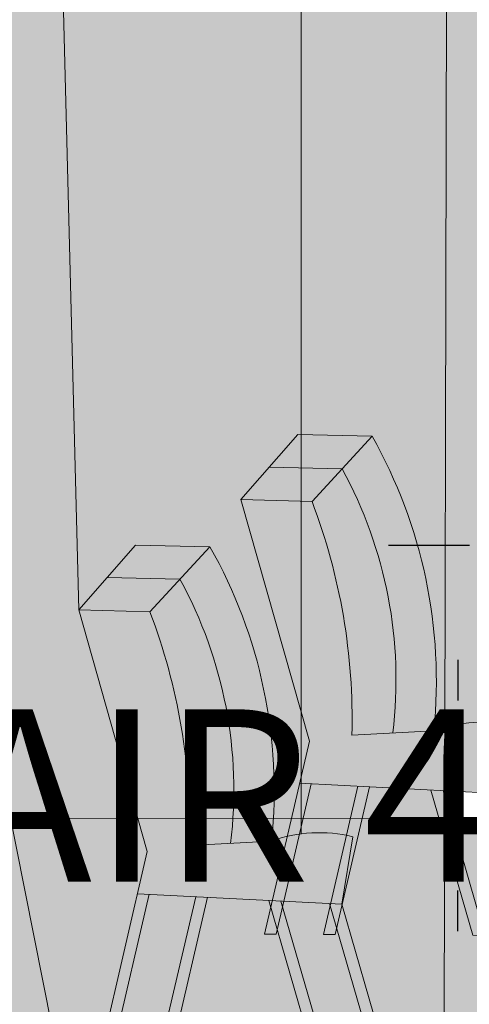
# Model space of a CAD drawing. Units: millimetres. Extents: x 11032 to 26788, y 3406 to 24505.
# Tile 6 of 78: x 15421 to 15812, y 7421 to 8278. Entities that reach past the tile are written whole.
import ezdxf

# ---------------------------------------------------------------- set-up
doc = ezdxf.new("R2010")
doc.units = ezdxf.units.MM
doc.header["$MEASUREMENT"] = 0
for name, color, linetype, lineweight in [('A-ANNO-DIMS', 2, 'Continuous', 18), ('A-FURN', 8, 'Continuous', 13), ('A-FURN-PATT', 8, 'Continuous', 13), ('A-GLAZ', 250, 'Continuous', 20), ('A-WALL-INTR', 8, 'Continuous', 18)]:
    doc.layers.add(name, color=color, linetype=linetype, lineweight=lineweight)
doc.layers.add('A-GLAZ-FRAM-PATT', color=250, linetype='Continuous', lineweight=13, true_color=0x262627)
doc.layers.add('A-WALL-INTR-PATT', color=251, linetype='Continuous', lineweight=13, true_color=0x6c6b6a)
doc.styles.get("Standard").update_dxf_attribs({"font": 'arial.ttf'})
doc.dimstyles.get("Standard").update_dxf_attribs({"dimtxt": 150, "dimasz": 100, "dimexe": 10, "dimexo": 5, "dimgap": 5, "dimtad": 0, "dimtih": 1, "dimtoh": 1, "dimdec": 0, "dimzin": 0, "dimdsep": 46, "dimtxsty": 'Standard', "dimcen": 0.09, "dimadec": 0, "dimazin": 0, "dimtfac": 1, "dimtdec": 0, "dimtofl": 0, "dimtmove": 0, "dimatfit": 3, "dimfxl": 1, "dimtolj": 1, "dimtzin": 0, "dimarcsym": 0})

# ---------------------------------------------------------------- blocks, each defined once
blk = doc.blocks.new('DINING-CHAIR-ELEV')
blk.add_line((228.68, 123.43), (51.04, 132.61))
for points in [[(0, 379.55), (49.45, 435.94), (114.12, 434.53)], [(61.18, 132.09), (30.79, 1.16), (20.53, 1.21), (59.55, 169.26), (0, 379.55), (61.9, 377.89)], [(111.9, 129.47), (82.06, 0.91), (71.8, 0.96), (101.76, 129.99)], [(165.28, 126.71), (201.76, 0.31), (212.19, 0.26), (175.85, 126.16)]]:
    blk.add_lwpolyline(points)
for points in [[(218.11, 123.98), (253.88, 0.05), (264.3, 0), (228.68, 123.43), (238.32, 182.18, 0.148451), (167.47, 178.33), (96.61, 174.48, 0.097012), (61.9, 377.89), (114.12, 434.53, -0.154833), (167.82, 178.46)], [(132.04, 176.4, 0.156877), (88.01, 406.21), (24.72, 407.74)]]:
    blk.add_lwpolyline(points, format="xyb")
blk = doc.blocks.new('*D16')
at = {"layer": 'A-ANNO-DIMS', "color": 0, "lineweight": -2, "transparency": 16777216}
for p, q in [((15741.74, 7821.05), (15812.13, 7821.05)), ((15802.13, 7721.05), (15802.13, 7685.69)), ((15802.13, 7485.11), (15802.13, 7520.47)), ((15741.74, 7385.11), (15812.13, 7385.11))]:
    blk.add_line(p, q, dxfattribs=at)
at = {"layer": 'A-ANNO-DIMS', "color": 0, "transparency": 16777216}
for points in [[(15785.47, 7721.05), (15818.8, 7721.05), (15802.13, 7821.05)], [(15785.47, 7485.11), (15818.8, 7485.11), (15802.13, 7385.11)]]:
    blk.add_solid(points, dxfattribs=at)
at = {"layer": 'Defpoints', "color": 0, "transparency": 16777216}
for p in [(15736.74, 7821.05), (15802.13, 7821.05), (15736.74, 7385.11)]:
    blk.add_point(p, dxfattribs=at)
at = {"layer": 'A-ANNO-DIMS', "color": 0, "transparency": 16777216, "insert": (15802.13, 7603.08), "char_height": 150, "attachment_point": 5}
blk.add_mtext('\\A1;CHAIR 436 TYP.', dxfattribs=at)
blk = doc.blocks.new('*D17')
at = {"layer": 'A-ANNO-DIMS', "color": 0, "lineweight": -2, "transparency": 16777216}
for p, q in [((15472.44, 7380.11), (15472.44, 7309.72)), ((15736.74, 7380.11), (15736.74, 7309.72)), ((15572.44, 7319.72), (15636.74, 7319.72)), ((15736.74, 7319.72), (15836.74, 7319.72))]:
    blk.add_line(p, q, dxfattribs=at)
at = {"layer": 'A-ANNO-DIMS', "color": 0, "transparency": 16777216}
for points in [[(15572.44, 7336.38), (15572.44, 7303.05), (15472.44, 7319.72)], [(15636.74, 7336.38), (15636.74, 7303.05), (15736.74, 7319.72)]]:
    blk.add_solid(points, dxfattribs=at)
at = {"layer": 'Defpoints', "color": 0, "transparency": 16777216}
for p in [(15472.44, 7385.11), (15736.74, 7385.11), (15736.74, 7319.72)]:
    blk.add_point(p, dxfattribs=at)
at = {"layer": 'A-ANNO-DIMS', "color": 0, "transparency": 16777216, "insert": (16266.37, 7319.72), "char_height": 150, "attachment_point": 5}
blk.add_mtext('\\A1;264 TYP.', dxfattribs=at)
blk = doc.blocks.new('*D36')
at = {"layer": 'A-ANNO-DIMS', "color": 0, "lineweight": -2, "transparency": 16777216}
for p, q in [((12301.26, 17115.89), (12301.26, 24416.86)), ((25397.4, 4466.4), (25397.4, 24416.86)), ((12401.26, 24406.86), (18569.2, 24406.86)), ((25297.4, 24406.86), (19129.47, 24406.86))]:
    blk.add_line(p, q, dxfattribs=at)
at = {"layer": 'A-ANNO-DIMS', "color": 0, "transparency": 16777216}
for points in [[(12401.26, 24423.52), (12401.26, 24390.19), (12301.26, 24406.86)], [(25297.4, 24423.52), (25297.4, 24390.19), (25397.4, 24406.86)]]:
    blk.add_solid(points, dxfattribs=at)
at = {"layer": 'Defpoints', "color": 0, "transparency": 16777216}
for p in [(25397.4, 24406.86), (12301.26, 17110.89), (25397.4, 4461.4)]:
    blk.add_point(p, dxfattribs=at)
at = {"layer": 'A-ANNO-DIMS', "color": 0, "transparency": 16777216, "insert": (18849.33, 24406.86), "char_height": 150, "attachment_point": 5}
blk.add_mtext('\\A1;13096', dxfattribs=at)
blk = doc.blocks.new('*D37')
at = {"layer": 'A-ANNO-DIMS', "color": 0, "lineweight": -2, "transparency": 16777216}
for p, q in [((18087.74, 23450.36), (11334.76, 23450.36)), ((11344.76, 23350.36), (11344.76, 14037.46)), ((11344.76, 4561.4), (11344.76, 13874.29)), ((12927.66, 4461.4), (11334.76, 4461.4))]:
    blk.add_line(p, q, dxfattribs=at)
at = {"layer": 'A-ANNO-DIMS', "color": 0, "transparency": 16777216}
for points in [[(11328.1, 23350.36), (11361.43, 23350.36), (11344.76, 23450.36)], [(11328.1, 4561.4), (11361.43, 4561.4), (11344.76, 4461.4)]]:
    blk.add_solid(points, dxfattribs=at)
at = {"layer": 'Defpoints', "color": 0, "transparency": 16777216}
for p in [(11344.76, 23450.36), (18092.74, 23450.36), (12932.66, 4461.4)]:
    blk.add_point(p, dxfattribs=at)
at = {"layer": 'A-ANNO-DIMS', "color": 0, "transparency": 16777216, "insert": (11344.76, 13955.88), "char_height": 150, "attachment_point": 5}
blk.add_mtext('\\A1;18989', dxfattribs=at)
blk = doc.blocks.new('*D49')
at = {"layer": 'A-ANNO-DIMS', "color": 0, "lineweight": -2, "transparency": 16777216}
for p, q in [((17953.45, 10206.41), (17953.45, 3494.9)), ((14996.4, 6406.4), (14996.4, 3494.9)), ((15096.4, 3504.9), (16244.67, 3504.9)), ((17853.45, 3504.9), (16705.18, 3504.9))]:
    blk.add_line(p, q, dxfattribs=at)
at = {"layer": 'A-ANNO-DIMS', "color": 0, "transparency": 16777216}
for points in [[(15096.4, 3521.57), (15096.4, 3488.23), (14996.4, 3504.9)], [(17853.45, 3521.57), (17853.45, 3488.23), (17953.45, 3504.9)]]:
    blk.add_solid(points, dxfattribs=at)
at = {"layer": 'Defpoints', "color": 0, "transparency": 16777216}
for p in [(17953.45, 10211.41), (14996.4, 6411.4), (17953.45, 3504.9)]:
    blk.add_point(p, dxfattribs=at)
at = {"layer": 'A-ANNO-DIMS', "color": 0, "transparency": 16777216, "insert": (16474.93, 3504.9), "char_height": 150, "attachment_point": 5}
blk.add_mtext('\\A1;2957', dxfattribs=at)
blk = doc.blocks.new('*D57')
at = {"layer": 'A-ANNO-DIMS', "color": 0, "lineweight": -2, "transparency": 16777216}
for p, q in [((14994.7, 7266.4), (14994.7, 24416.86)), ((20894.7, 7266.4), (20894.7, 24416.86)), ((15094.7, 24406.86), (17715.98, 24406.86)), ((20794.7, 24406.86), (18173.42, 24406.86))]:
    blk.add_line(p, q, dxfattribs=at)
at = {"layer": 'A-ANNO-DIMS', "color": 0, "transparency": 16777216}
for points in [[(15094.7, 24423.52), (15094.7, 24390.19), (14994.7, 24406.86)], [(20794.7, 24423.52), (20794.7, 24390.19), (20894.7, 24406.86)]]:
    blk.add_solid(points, dxfattribs=at)
at = {"layer": 'Defpoints', "color": 0, "transparency": 16777216}
for p in [(20894.7, 24406.86), (14994.7, 7261.4), (20894.7, 7261.4)]:
    blk.add_point(p, dxfattribs=at)
at = {"layer": 'A-ANNO-DIMS', "color": 0, "transparency": 16777216, "insert": (17944.7, 24406.86), "char_height": 150, "attachment_point": 5}
blk.add_mtext('\\A1;5900', dxfattribs=at)
blk = doc.blocks.new('*D60')
at = {"layer": 'A-ANNO-DIMS', "color": 0, "lineweight": -2, "transparency": 16777216}
for p, q in [((14994.7, 7266.4), (14994.7, 24416.86)), ((16344.7, 7266.4), (16344.7, 24416.86)), ((15094.7, 24406.86), (15448.04, 24406.86)), ((16244.7, 24406.86), (15891.36, 24406.86))]:
    blk.add_line(p, q, dxfattribs=at)
at = {"layer": 'A-ANNO-DIMS', "color": 0, "transparency": 16777216}
for points in [[(15094.7, 24423.52), (15094.7, 24390.19), (14994.7, 24406.86)], [(16244.7, 24423.52), (16244.7, 24390.19), (16344.7, 24406.86)]]:
    blk.add_solid(points, dxfattribs=at)
at = {"layer": 'Defpoints', "color": 0, "transparency": 16777216}
for p in [(16344.7, 24406.86), (14994.7, 7261.4), (16344.7, 7261.4)]:
    blk.add_point(p, dxfattribs=at)
at = {"layer": 'A-ANNO-DIMS', "color": 0, "transparency": 16777216, "insert": (15669.7, 24406.86), "char_height": 150, "attachment_point": 5}
blk.add_mtext('\\A1;1350', dxfattribs=at)
blk = doc.blocks.new('*D69')
at = {"layer": 'A-ANNO-DIMS', "color": 0, "lineweight": -2, "transparency": 16777216}
for p, q in [((13956.97, 9937.95), (14056.97, 9937.95)), ((14056.97, 9937.95), (15432.5, 8990.95)), ((17944.61, 7261.4), (17944.79, 7261.4)), ((17944.7, 7261.31), (17944.7, 7261.49))]:
    blk.add_line(p, q, dxfattribs=at)
at = {"layer": 'A-ANNO-DIMS', "color": 0, "transparency": 16777216}
blk.add_solid([(15441.95, 9004.68), (15423.05, 8977.22), (15514.87, 8934.24)], dxfattribs=at)
at = {"layer": 'Defpoints', "color": 0, "transparency": 16777216}
for p in [(15514.87, 8934.24), (17944.7, 7261.4)]:
    blk.add_point(p, dxfattribs=at)
at = {"layer": 'A-ANNO-DIMS', "color": 0, "transparency": 16777216, "insert": (13494.04, 9937.95), "char_height": 150, "attachment_point": 5}
blk.add_mtext('\\A1;2X R2950', dxfattribs=at)

msp = doc.modelspace()

# ---------------------------------------------------------------- hatches: boundary and pattern name
at = {"layer": 'A-FURN-PATT'}
h = msp.add_hatch(color=256, dxfattribs=at)
h.set_gradient(color1=(153, 27, 30), color2=(153, 38, 0), name='SPHERICAL')
h.paths.add_polyline_path([(15534.344, 7763), (15472.44, 7764.657), (15531.986, 7554.365), (15523.479, 7517.719), (15640.736, 7511.661), (15653.713, 7567.556, 0.0295203), (15639.906, 7563.436), (15569.055, 7559.583, 0.0970121)], flags=16)
h.paths.add_polyline_path([(15560.453, 7791.32), (15534.344, 7763, -0.0970121), (15569.055, 7559.583), (15604.48, 7561.509, 0.1568775)], flags=16)
h.paths.add_polyline_path([(15586.562, 7819.64), (15560.453, 7791.32, -0.1568775), (15604.48, 7561.509), (15640.246, 7563.454, 0.154898)], flags=17)
h.paths.add_polyline_path([(15560.453, 7791.32), (15497.165, 7792.851), (15472.44, 7764.657), (15534.344, 7763)], flags=16)
h.paths.add_polyline_path([(15586.562, 7819.64), (15521.889, 7821.046), (15497.165, 7792.851), (15560.453, 7791.32)], flags=17)
h.paths.add_polyline_path([(15790.874, 7662.689, 0.021469), (15780.879, 7659.53), (15710.028, 7655.677, 0.0970121), (15675.317, 7859.094), (15665.772, 7859.35), (15665.799, 7675.745), (15672.959, 7650.459), (15665.807, 7619.654), (15665.808, 7613.744), (15790.755, 7607.288)], flags=17)
h.paths.add_polyline_path([(15665.772, 7859.35), (15613.413, 7860.751), (15665.799, 7675.745)], flags=16)
h.paths.add_polyline_path([(15701.426, 7887.414), (15665.767, 7888.277), (15665.772, 7859.35), (15675.317, 7859.094)], flags=16)
h.paths.add_polyline_path([(15727.534, 7915.735), (15665.763, 7917.077), (15665.767, 7888.277), (15701.426, 7887.414)], flags=17)
h.paths.add_polyline_path([(15665.763, 7917.077), (15662.862, 7917.14), (15638.137, 7888.946), (15665.767, 7888.277)], flags=17)
h.paths.add_polyline_path([(15665.767, 7888.277), (15638.137, 7888.946), (15613.413, 7860.751), (15665.772, 7859.35)], flags=16)
h.paths.add_polyline_path([(15701.426, 7887.414), (15675.317, 7859.094, -0.0970121), (15710.028, 7655.677), (15745.453, 7657.604, 0.1568775)], flags=16)
h.paths.add_polyline_path([(15844.495, 7664.925), (15844.384, 7864.461), (15821.312, 7945.94), (15870.762, 8002.329), (15935.434, 8000.923, -0.1195917), (15991.005, 7804.617), (16002.667, 7804.617), (16022.264, 7889.032), (15962.718, 8099.323), (16024.622, 8097.666), (16076.839, 8154.307, -0.1548334), (16130.535, 7898.229, -0.1476694), (16201.035, 7901.954), (16191.395, 7843.208), (16202.533, 7804.617), (16299.12, 7804.617), (16297.929, 7808.825), (16347.378, 7865.214), (16412.05, 7863.808, -0.0295496), (16434.494, 7817.915), (16458.237, 7920.19), (16398.691, 8130.481), (16460.595, 8128.825), (16512.813, 8185.465, -0.1548334), (16566.508, 7929.387, -0.1476694), (16637.008, 7933.112), (16627.369, 7874.366), (16647.499, 7804.617), (16830.506, 7804.617), (16830.506, 7793.515), (16650.704, 7793.515), (16662.994, 7750.932), (16652.571, 7750.983), (16640.296, 7793.515), (16490.425, 7793.515), (16480.749, 7751.837), (16470.495, 7751.888), (16480.159, 7793.515), (16443.833, 7793.515, -0.1094051), (16465.746, 7607.731, -0.1476694), (16536.246, 7611.456), (16526.606, 7552.71), (16562.232, 7429.275), (16551.809, 7429.327), (16516.041, 7553.255), (16473.778, 7555.439), (16510.116, 7429.534), (16499.693, 7429.586), (16463.212, 7555.985), (16409.833, 7558.743), (16379.987, 7430.181), (16369.733, 7430.232), (16394.704, 7537.793), (16394.704, 7559.524), (16359.112, 7561.363), (16328.717, 7430.435), (16318.463, 7430.486), (16344.704, 7543.521), (16344.704, 7643.635), (16302.264, 7793.515), (16205.738, 7793.515), (16227.021, 7719.773), (16216.598, 7719.825), (16195.329, 7793.515), (16153.697, 7793.515), (16174.905, 7720.032), (16164.482, 7720.084), (16143.289, 7793.515), (16061.685, 7793.515), (16051.641, 7750.248, -0.0167144), (16059.629, 7748.571), (16049.99, 7689.825), (16085.615, 7566.39), (16075.192, 7566.442), (16039.424, 7690.371), (15997.161, 7692.554), (16033.5, 7566.649), (16023.077, 7566.701), (15986.595, 7693.1), (15933.216, 7695.858), (15903.371, 7567.296), (15893.116, 7567.347), (15923.072, 7696.382), (15882.495, 7698.478), (15852.409, 7568.882), (15877.716, 7481.201), (15867.293, 7481.253), (15842.372, 7567.599), (15841.846, 7567.602), (15842.08, 7568.609), (15831.524, 7605.182), (15790.755, 7607.288), (15790.744, 7602.228), (15825.6, 7481.46), (15815.177, 7481.512), (15778.696, 7607.911), (15725.317, 7610.669), (15701.389, 7507.6), (15736.743, 7385.107), (15726.32, 7385.159), (15696.749, 7487.614), (15695.471, 7482.107), (15685.217, 7482.158), (15691.06, 7507.327), (15690.552, 7509.088), (15650.881, 7511.137), (15649.743, 7506.234), (15684.627, 7385.366), (15674.204, 7385.418), (15645.103, 7486.248), (15644.2, 7482.362), (15633.946, 7482.413), (15639.413, 7505.961), (15637.723, 7511.817), (15584.344, 7514.575), (15554.498, 7386.013), (15544.244, 7386.064), (15574.2, 7515.099), (15533.623, 7517.195), (15503.228, 7386.268), (15492.974, 7386.319), (15531.986, 7554.365), (15472.44, 7764.657), (15497.165, 7792.851), (15521.889, 7821.046), (15586.562, 7819.64, -0.1548334), (15640.257, 7563.563, -0.0287549), (15653.713, 7567.556), (15665.807, 7619.654), (15665.799, 7675.745), (15613.413, 7860.751), (15638.137, 7888.946), (15662.862, 7917.14), (15665.763, 7917.077), (15727.534, 7915.735, -0.1548334), (15781.23, 7659.657, -0.1322263)])
h = msp.add_hatch(color=256, dxfattribs=at)
h.set_gradient(color1=(153, 27, 30), color2=(153, 38, 0), name='SPHERICAL')
h.paths.add_polyline_path([(15710.028, 7655.677), (15745.453, 7657.604, 0.1568775), (15701.426, 7887.414), (15675.317, 7859.094, -0.0970121)], flags=16)
h.paths.add_polyline_path([(15790.755, 7607.288), (15790.874, 7662.689, 0.021469), (15780.879, 7659.53), (15710.028, 7655.677, 0.0970121), (15675.317, 7859.094), (15665.772, 7859.35), (15665.799, 7675.745), (15672.959, 7650.459), (15665.807, 7619.654), (15665.808, 7613.744)], flags=17)
h.paths.add_polyline_path([(15653.713, 7567.556), (15665.807, 7619.654), (15665.799, 7675.745), (15613.413, 7860.751), (15662.862, 7917.14), (15727.534, 7915.735, -0.1548334), (15781.23, 7659.657, -0.1322263), (15844.495, 7664.925), (15844.384, 7864.461), (15821.312, 7945.94), (15883.216, 7944.283), (15935.434, 8000.923, -0.1195917), (15991.005, 7804.617), (16002.667, 7804.617), (16022.264, 7889.032), (15962.718, 8099.323), (16024.622, 8097.666), (16076.839, 8154.307, -0.1548334), (16130.535, 7898.229, -0.1476694), (16201.035, 7901.954), (16191.395, 7843.208), (16202.533, 7804.617), (16830.506, 7804.617), (16830.506, 7793.515), (16205.738, 7793.515), (16227.021, 7719.773), (16216.598, 7719.825), (16195.329, 7793.515), (16153.697, 7793.515), (16174.905, 7720.032), (16164.482, 7720.084), (16143.289, 7793.515), (16061.685, 7793.515), (16051.641, 7750.248, -0.0167144), (16059.629, 7748.571), (16049.99, 7689.825), (16085.615, 7566.39), (16075.192, 7566.442), (16039.424, 7690.371), (15997.161, 7692.554), (16033.5, 7566.649), (16023.077, 7566.701), (15986.595, 7693.1), (15933.216, 7695.858), (15903.371, 7567.296), (15893.116, 7567.347), (15923.072, 7696.382), (15882.495, 7698.478), (15852.409, 7568.882), (15877.716, 7481.201), (15867.293, 7481.253), (15842.372, 7567.599), (15841.846, 7567.602), (15842.08, 7568.609), (15831.524, 7605.182), (15790.755, 7607.288), (15790.744, 7602.228), (15825.6, 7481.46), (15815.177, 7481.512), (15778.696, 7607.911), (15725.317, 7610.669), (15701.389, 7507.6), (15736.743, 7385.107), (15726.32, 7385.159), (15696.749, 7487.614), (15695.471, 7482.107), (15685.217, 7482.158), (15705.262, 7568.502, 0.0841685), (15664.448, 7569.579), (15644.2, 7482.362), (15633.946, 7482.413), (15653.713, 7567.556, 0.0295203), (15639.906, 7563.436), (15569.055, 7559.583, 0.0970121), (15534.344, 7763), (15472.44, 7764.657), (15521.889, 7821.046), (15586.562, 7819.64, -0.1548334), (15640.257, 7563.563, -0.0287549)])
h = msp.add_hatch(color=256, dxfattribs=at)
h.set_gradient(color1=(153, 27, 30), color2=(153, 38, 0), name='SPHERICAL')
h.paths.add_polyline_path([(15675.317, 7859.094), (15665.772, 7859.35), (15665.799, 7675.745), (15672.959, 7650.459), (15665.807, 7619.654), (15665.808, 7613.744), (15790.755, 7607.288), (15790.874, 7662.689, 0.021469), (15780.879, 7659.53), (15710.028, 7655.677, 0.0970121)])
h.paths.add_polyline_path([(15710.028, 7655.677), (15745.453, 7657.604, 0.1568775), (15701.426, 7887.414), (15675.317, 7859.094, -0.0970121)])
h = msp.add_hatch(color=256, dxfattribs=at)
h.set_gradient(color1=(153, 27, 30), color2=(153, 38, 0), name='SPHERICAL')
h.paths.add_polyline_path([(15534.344, 7763), (15472.44, 7764.657), (15531.986, 7554.365), (15523.479, 7517.719), (15640.736, 7511.661), (15653.713, 7567.556, 0.0295203), (15639.906, 7563.436), (15569.055, 7559.583, 0.0970121)])
h.paths.add_polyline_path([(15560.453, 7791.32), (15534.344, 7763, -0.0970121), (15569.055, 7559.583), (15604.48, 7561.509, 0.1568775)])
at = {"layer": 'A-GLAZ-FRAM-PATT'}
h = msp.add_hatch(color=256, dxfattribs=at)
h.paths.add_polyline_path([(17944.704, 7311.399), (16344.704, 7311.399), (16344.704, 7261.399), (17944.704, 7261.399)], flags=17)
h.paths.add_polyline_path([(16344.704, 7311.399), (15045.135, 7311.399, -0.9829047), (20844.273, 7311.399), (19544.704, 7311.399), (19544.704, 7261.399), (20894.704, 7261.399, 0.5148441), (16985.951, 10051.255, 0.3202679), (14994.704, 7261.399), (16344.704, 7261.399)])
h.paths.add_polyline_path([(18744.704, 7311.399), (17944.704, 7311.399), (17944.704, 7261.399), (18744.704, 7261.399)], flags=17)
h.paths.add_polyline_path([(19544.704, 7311.399), (18744.704, 7311.399), (18744.704, 7261.399), (19544.704, 7261.399)], flags=17)
h.paths.add_polyline_path([(18694.704, 7361.399), (17994.704, 7361.399), (17994.704, 7311.399), (18694.704, 7311.399)], flags=17)
h.paths.add_polyline_path([(18744.704, 7361.399), (18694.704, 7361.399), (18694.704, 7311.399), (18744.704, 7311.399)], flags=17)
h.paths.add_polyline_path([(17194.704, 7361.399), (17144.704, 7361.399), (17144.704, 7311.399), (17194.704, 7311.399)], flags=17)
h.paths.add_polyline_path([(17431.432, 7361.399), (17194.704, 7361.399), (17194.704, 7311.399), (17431.699, 7311.399)], flags=17)
h.paths.add_polyline_path([(17894.704, 7361.399), (17431.432, 7361.399), (17431.699, 7311.399), (17894.704, 7311.399)], flags=17)
h.paths.add_polyline_path([(17944.704, 7361.399), (17894.704, 7361.399), (17894.704, 7311.399), (17944.704, 7311.399)], flags=17)
h.paths.add_polyline_path([(17994.704, 7361.399), (17944.704, 7361.399), (17944.704, 7311.399), (17994.704, 7311.399)], flags=17)
at = {"layer": 'A-WALL-INTR-PATT'}
for points in [[(15843.607, 9260.247, 0.0062633), (15794.195, 9206.987), (15790.874, 7662.689, -0.1112179), (15844.495, 7664.925), (15844.384, 7864.461), (15821.312, 7945.94), (15844.324, 7972.181)], [(15794.195, 9206.987, 0.0171928), (15665.595, 9054.627), (15665.763, 7917.077), (15727.534, 7915.735, -0.1548334), (15781.23, 7659.657, -0.0207039), (15790.874, 7662.689)], [(15665.595, 9054.627, 0.0332657), (15447.906, 8736.527), (15472.44, 7764.657), (15521.889, 7821.046), (15586.562, 7819.64, -0.1548334), (15640.257, 7563.563, -0.0287549), (15653.713, 7567.556), (15665.807, 7619.654), (15665.799, 7675.745), (15613.413, 7860.751), (15662.862, 7917.14), (15665.763, 7917.077)], [(15447.906, 8736.527, 0.0271717), (15302.659, 8457.059), (15381.661, 7740.545), (15467.334, 7311.399), (15790.119, 7311.399), (15790.667, 7566.433), (15778.696, 7607.911), (15725.317, 7610.669), (15701.389, 7507.6), (15736.743, 7385.107), (15726.32, 7385.159), (15696.749, 7487.614), (15695.471, 7482.107), (15685.217, 7482.158), (15691.06, 7507.327), (15690.552, 7509.088), (15650.881, 7511.137), (15649.743, 7506.234), (15684.627, 7385.366), (15674.204, 7385.418), (15645.103, 7486.248), (15644.2, 7482.362), (15633.946, 7482.413), (15639.413, 7505.961), (15637.723, 7511.817), (15584.344, 7514.575), (15554.498, 7386.013), (15544.244, 7386.064), (15574.2, 7515.099), (15533.623, 7517.195), (15503.228, 7386.268), (15492.974, 7386.319), (15531.986, 7554.365), (15472.44, 7764.657)]]:
    msp.add_hatch(color=256, dxfattribs=at).paths.add_polyline_path(points)
h = msp.add_hatch(color=256, dxfattribs=at)
h.paths.add_polyline_path([(15302.659, 8457.059, 0.0281002), (15185.248, 8153.253), (15233.282, 7717.599), (15314.374, 7311.399), (15467.334, 7311.399), (15381.661, 7740.545)])
h.paths.add_polyline_path([(16344.704, 7543.521), (16344.704, 7643.635), (16302.264, 7793.515), (16205.738, 7793.515), (16227.021, 7719.773), (16216.598, 7719.825), (16195.329, 7793.515), (16153.697, 7793.515), (16174.905, 7720.032), (16164.482, 7720.084), (16143.289, 7793.515), (16061.685, 7793.515), (16051.641, 7750.248, -0.0167144), (16059.629, 7748.571), (16049.99, 7689.825), (16085.615, 7566.39), (16075.192, 7566.442), (16039.424, 7690.371), (15997.161, 7692.554), (16033.5, 7566.649), (16023.077, 7566.701), (15986.595, 7693.1), (15933.216, 7695.858), (15903.371, 7567.296), (15893.116, 7567.347), (15923.072, 7696.382), (15882.495, 7698.478), (15852.409, 7568.882), (15877.716, 7481.201), (15867.293, 7481.253), (15844.553, 7560.041), (15844.691, 7311.399), (16344.704, 7311.399), (16344.704, 7499.3), (16328.717, 7430.435), (16318.463, 7430.486)])
h.paths.add_polyline_path([(16742.983, 7793.515), (16650.704, 7793.515), (16662.994, 7750.932), (16652.571, 7750.983), (16640.296, 7793.515), (16598.663, 7793.515), (16610.879, 7751.191), (16600.455, 7751.242), (16588.255, 7793.515), (16490.425, 7793.515), (16480.749, 7751.837), (16470.495, 7751.888), (16480.159, 7793.515), (16443.833, 7793.515, -0.1094051), (16465.746, 7607.731, -0.1476694), (16536.246, 7611.456), (16526.606, 7552.71), (16562.232, 7429.275), (16551.809, 7429.327), (16516.041, 7553.255), (16473.778, 7555.439), (16510.116, 7429.534), (16499.693, 7429.586), (16463.212, 7555.985), (16409.833, 7558.743), (16394.704, 7493.572), (16394.704, 7361.399), (16744.704, 7361.399)])
h.paths.add_polyline_path([(17094.704, 8239.696), (16741.207, 8239.696), (16742.939, 7804.617), (16768.057, 7804.617), (16785.352, 7864.542), (16775.713, 7923.288, -0.1476694), (16846.212, 7919.563, -0.1548334), (16899.908, 8175.64), (16964.58, 8177.046), (17014.03, 8120.657), (16954.484, 7910.365), (16972.017, 7834.84), (16977.75, 7834.965), (17027.199, 7778.576), (16967.653, 7568.284), (17006.665, 7400.238), (16996.411, 7400.187), (16966.016, 7531.114), (16925.439, 7529.018), (16955.395, 7399.983), (16945.141, 7399.932), (16915.295, 7528.494), (16861.916, 7525.736), (16825.435, 7399.337), (16815.012, 7399.285), (16851.35, 7525.19), (16809.087, 7523.007), (16773.319, 7399.078), (16762.896, 7399.026), (16798.521, 7522.461), (16788.882, 7581.207, -0.1476694), (16859.382, 7577.482, -0.1528132), (16911.41, 7830.579), (16902.125, 7870.575), (16848.746, 7867.817), (16830.506, 7804.617), (16830.506, 7793.515), (16827.302, 7793.515), (16812.265, 7741.418), (16801.842, 7741.366), (16816.893, 7793.515), (16775.261, 7793.515), (16760.15, 7741.159), (16749.727, 7741.107), (16764.853, 7793.515), (16742.983, 7793.515), (16744.704, 7361.399), (17094.704, 7361.399)])
h.paths.add_polyline_path([(18950.929, 7931.023), (19015.601, 7932.429), (19065.05, 7876.04), (19005.504, 7665.748), (19014.012, 7629.102, -0.129191), (19069.892, 7841.762), (19134.564, 7843.167), (19168.958, 7803.946), (19202.145, 7841.791), (19246.92, 7840.817), (19212.932, 7960.847), (19262.382, 8017.236), (19327.054, 8015.831, -0.134919), (19382.824, 7793.43), (19562.845, 7793.43, -0.1257757), (19618.686, 8000.275), (19683.358, 8001.68), (19732.808, 7945.291), (19689.807, 7793.43), (19753.644, 7793.43, -0.0966843), (19805.964, 7950.707), (19870.637, 7952.112), (19920.086, 7895.723), (19891.121, 7793.43), (20039.255, 7793.43, -0.0897865), (20089.9, 7938.993), (20154.572, 7940.399), (20204.021, 7884.01), (20144.475, 7673.718), (20152.983, 7637.072, -0.1476694), (20223.483, 7633.347, -0.1548334), (20277.178, 7889.425), (20341.85, 7890.831), (20391.3, 7834.441), (20331.754, 7624.15), (20370.766, 7456.103), (20360.512, 7456.052), (20330.117, 7586.98), (20289.54, 7584.884), (20319.496, 7455.848), (20309.241, 7455.797), (20279.396, 7584.359), (20226.017, 7581.602), (20189.536, 7455.202), (20179.112, 7455.151), (20215.451, 7581.056), (20173.188, 7578.872), (20169.478, 7566.018), (20183.488, 7505.671), (20173.234, 7505.62), (20163.789, 7546.305), (20137.42, 7454.943), (20126.997, 7454.892), (20159.149, 7566.291), (20142.839, 7636.548), (20102.261, 7634.452), (20132.217, 7505.417), (20121.963, 7505.366), (20092.117, 7633.928), (20038.738, 7631.17), (20002.257, 7504.771), (19991.834, 7504.719), (20028.172, 7630.624), (19985.91, 7628.44), (19950.141, 7504.512), (19939.718, 7504.46), (19975.344, 7627.895), (19965.704, 7686.641, -0.1476694), (20036.204, 7682.916, -0.0576487), (20037.659, 7782.328), (19887.977, 7782.328), (19860.54, 7685.431), (19899.552, 7517.385), (19889.298, 7517.334), (19858.903, 7648.261), (19818.326, 7646.165), (19848.282, 7517.13), (19838.028, 7517.079), (19808.182, 7645.641), (19754.803, 7642.883), (19718.322, 7516.484), (19707.899, 7516.432), (19744.237, 7642.337), (19701.974, 7640.154), (19698.264, 7627.3), (19712.274, 7566.953), (19702.02, 7566.902), (19692.575, 7607.587), (19666.206, 7516.225), (19655.783, 7516.173), (19687.935, 7627.573), (19671.625, 7697.83), (19631.048, 7695.733), (19661.003, 7566.698), (19650.749, 7566.647), (19620.903, 7695.209), (19567.524, 7692.451), (19531.043, 7566.052), (19520.62, 7566), (19556.959, 7691.905), (19514.696, 7689.722), (19478.928, 7565.793), (19468.505, 7565.741), (19473, 7581.318), (19466.812, 7581.349), (19431.044, 7705.278), (19388.781, 7707.461), (19425.12, 7581.556), (19414.696, 7581.608), (19378.215, 7708.007), (19324.836, 7710.765), (19318.877, 7685.094, -0.0584523), (19320.513, 7584.307, -0.1476694), (19391.013, 7588.032), (19381.373, 7529.286), (19416.999, 7405.852), (19406.576, 7405.903), (19370.808, 7529.832), (19328.545, 7532.016), (19364.883, 7406.111), (19354.46, 7406.162), (19317.979, 7532.562), (19264.6, 7535.319), (19234.754, 7406.757), (19224.5, 7406.808), (19254.456, 7535.844), (19213.879, 7537.94), (19183.484, 7407.012), (19173.23, 7407.063), (19212.242, 7575.11), (19168.16, 7730.789), (19124.467, 7576.487), (19163.48, 7408.44), (19153.225, 7408.389), (19122.83, 7539.317), (19082.253, 7537.22), (19112.209, 7408.185), (19101.955, 7408.134), (19072.109, 7536.696), (19035.898, 7534.825), (19044.517, 7497.701), (19034.262, 7497.65), (19025.754, 7534.301), (19018.73, 7533.938), (18982.249, 7407.539), (18971.826, 7407.487), (19008.164, 7533.392), (18985.177, 7532.205), (18993.246, 7497.447), (18982.992, 7497.396), (18975.033, 7531.681), (18965.902, 7531.209), (18930.133, 7407.28), (18919.71, 7407.228), (18955.336, 7530.663), (18945.696, 7589.409, -0.0318483), (18960.996, 7592.142), (18953.146, 7625.958), (18899.767, 7623.2), (18863.286, 7496.801), (18852.863, 7496.749), (18889.201, 7622.654), (18846.938, 7620.47), (18811.17, 7496.542), (18800.747, 7496.49), (18836.373, 7619.924), (18826.733, 7678.67, -0.1476694), (18897.233, 7674.946, -0.1548334)], flags=16)
h = msp.add_hatch(color=256, dxfattribs=at)
h.set_gradient(color1=(254, 234, 185), color2=(254, 204, 102), name='CURVED')
h.paths.add_polyline_path([(15260.167, 7582.928), (15062.56, 7582.722, 0.023451), (15045.135, 7311.399), (15314.374, 7311.399)])
h.paths.add_polyline_path([(15413.095, 7583.087), (15260.167, 7582.928), (15314.374, 7311.399), (15467.334, 7311.399)])
h.paths.add_polyline_path([(15531.986, 7554.365), (15523.82, 7583.203), (15413.095, 7583.087), (15467.334, 7311.399), (15790.119, 7311.399), (15790.667, 7566.433), (15785.748, 7583.476), (15718.988, 7583.406), (15701.389, 7507.6), (15736.743, 7385.107), (15726.32, 7385.159), (15696.749, 7487.614), (15695.471, 7482.107), (15685.217, 7482.158), (15691.06, 7507.327), (15690.552, 7509.088), (15650.881, 7511.137), (15649.743, 7506.234), (15684.627, 7385.366), (15674.204, 7385.418), (15646.227, 7482.352), (15633.946, 7482.413), (15639.413, 7505.961), (15637.723, 7511.817), (15584.344, 7514.575), (15554.498, 7386.013), (15544.244, 7386.064), (15574.2, 7515.099), (15533.623, 7517.195), (15503.228, 7386.268), (15492.974, 7386.319)])
h.paths.add_polyline_path([(16344.704, 7499.3), (16328.717, 7430.435), (16318.463, 7430.486), (16344.704, 7543.521), (16344.704, 7584.059), (16080.595, 7583.783), (16085.615, 7566.39), (16075.192, 7566.442), (16070.19, 7583.773), (16028.57, 7583.729), (16033.5, 7566.649), (16023.077, 7566.701), (16018.165, 7583.718), (15907.156, 7583.603), (15903.371, 7567.296), (15893.116, 7567.347), (15896.888, 7583.592), (15855.814, 7583.549), (15852.409, 7568.882), (15877.716, 7481.201), (15867.293, 7481.253), (15844.553, 7560.041), (15844.691, 7311.399), (16344.704, 7311.399)])
h.paths.add_polyline_path([(15844.553, 7560.041), (15842.372, 7567.599), (15841.846, 7567.602), (15842.08, 7568.609), (15837.773, 7583.53), (15796.153, 7583.487), (15825.6, 7481.46), (15815.177, 7481.512), (15790.667, 7566.433), (15790.119, 7311.399), (15844.691, 7311.399)])
h.paths.add_polyline_path([(16394.704, 7493.572), (16379.987, 7430.181), (16369.733, 7430.232), (16394.704, 7537.793), (16394.704, 7559.524), (16359.112, 7561.363), (16344.704, 7499.3), (16344.704, 7311.399), (17144.704, 7311.399), (17144.704, 7584.893), (17094.704, 7584.841), (17094.704, 7361.399), (16394.704, 7361.399)])
h.paths.add_polyline_path([(17430.237, 7585.191), (17194.704, 7584.945), (17194.704, 7361.399), (17431.432, 7361.399)])
h.paths.add_polyline_path([(17894.704, 7585.675), (17748.458, 7585.522), (17754.673, 7563.99), (17744.25, 7564.042), (17738.053, 7585.511), (17696.433, 7585.468), (17702.557, 7564.249), (17692.134, 7564.301), (17686.028, 7585.457), (17577.175, 7585.344), (17572.428, 7564.896), (17562.174, 7564.947), (17566.907, 7585.333), (17525.833, 7585.29), (17521.158, 7565.151), (17510.903, 7565.202), (17515.565, 7585.28), (17430.237, 7585.191), (17431.432, 7361.399), (17894.704, 7361.399)])
h.paths.add_polyline_path([(18694.704, 7586.509), (18404.857, 7586.207), (18425.604, 7496.839), (18415.35, 7496.788), (18394.593, 7586.196), (18353.54, 7586.153), (18374.333, 7496.584), (18364.079, 7496.533), (18343.276, 7586.142), (18270.386, 7586.066), (18244.373, 7495.938), (18233.95, 7495.887), (18259.974, 7586.056), (18218.329, 7586.012), (18192.257, 7495.679), (18181.834, 7495.628), (18207.918, 7586.001), (17994.704, 7585.779), (17994.704, 7361.399), (18694.704, 7361.399)])
h.paths.add_polyline_path([(19317.979, 7532.562), (19264.6, 7535.319), (19234.754, 7406.757), (19224.5, 7406.808), (19254.456, 7535.844), (19213.879, 7537.94), (19183.484, 7407.012), (19173.23, 7407.063), (19212.242, 7575.11), (19208.862, 7587.045), (19127.433, 7586.96), (19124.467, 7576.487), (19163.48, 7408.44), (19153.225, 7408.389), (19122.83, 7539.317), (19082.253, 7537.22), (19112.209, 7408.185), (19101.955, 7408.134), (19072.109, 7536.696), (19035.898, 7534.825), (19044.517, 7497.701), (19034.262, 7497.65), (19025.754, 7534.301), (19018.73, 7533.938), (18982.249, 7407.539), (18971.826, 7407.487), (19008.164, 7533.392), (18985.177, 7532.205), (18993.246, 7497.447), (18982.992, 7497.396), (18975.033, 7531.681), (18965.902, 7531.209), (18930.133, 7407.28), (18919.71, 7407.228), (18955.336, 7530.663), (18946.129, 7586.771), (18889.236, 7586.712), (18863.286, 7496.801), (18852.863, 7496.749), (18878.825, 7586.701), (18837.179, 7586.657), (18811.17, 7496.542), (18800.747, 7496.49), (18826.768, 7586.647), (18794.704, 7586.613), (18794.704, 7361.399), (19494.704, 7361.399), (19494.704, 7587.343), (19485.145, 7587.333), (19478.928, 7565.793), (19468.505, 7565.741), (19473, 7581.318), (19466.812, 7581.349), (19465.091, 7587.312), (19423.471, 7587.269), (19425.12, 7581.556), (19414.696, 7581.608), (19413.066, 7587.258), (19390.882, 7587.235), (19381.373, 7529.286), (19416.999, 7405.852), (19406.576, 7405.903), (19370.808, 7529.832), (19328.545, 7532.016), (19364.883, 7406.111), (19354.46, 7406.162)])
h.paths.add_polyline_path([(19990.261, 7587.86), (19974.192, 7587.843), (19950.141, 7504.512), (19939.718, 7504.46), (19963.781, 7587.832), (19883.217, 7587.748), (19899.552, 7517.385), (19889.298, 7517.334), (19872.954, 7587.737), (19831.9, 7587.695), (19848.282, 7517.13), (19838.028, 7517.079), (19821.637, 7587.684), (19738.846, 7587.598), (19718.322, 7516.484), (19707.899, 7516.432), (19728.435, 7587.587), (19707.489, 7587.565), (19712.274, 7566.953), (19702.02, 7566.902), (19697.225, 7587.554), (19686.79, 7587.543), (19666.206, 7516.225), (19655.783, 7516.173), (19676.379, 7587.532), (19656.172, 7587.511), (19661.003, 7566.698), (19650.749, 7566.647), (19645.908, 7587.501), (19544.704, 7587.395), (19544.704, 7311.399), (19990.261, 7311.399)])
h.paths.add_polyline_path([(20190.261, 7455.206), (20179.112, 7455.151), (20190.261, 7493.779), (20190.261, 7579.754), (20173.188, 7578.872), (20169.478, 7566.018), (20183.488, 7505.671), (20173.234, 7505.62), (20163.789, 7546.305), (20137.42, 7454.943), (20126.997, 7454.892), (20159.149, 7566.291), (20154.102, 7588.03), (20113.048, 7587.988), (20132.217, 7505.417), (20121.963, 7505.366), (20102.785, 7587.977), (20026.249, 7587.897), (20002.257, 7504.771), (19990.261, 7504.711), (19990.261, 7311.399), (20190.261, 7311.399)])
h.paths.add_polyline_path([(20340.261, 7543.283), (20330.117, 7586.98), (20289.54, 7584.884), (20319.496, 7455.848), (20309.241, 7455.797), (20279.396, 7584.359), (20226.017, 7581.602), (20190.261, 7457.717), (20190.261, 7311.399), (20340.261, 7311.399)])
h.paths.add_polyline_path([(20826.171, 7588.731), (20340.261, 7588.225), (20340.261, 7587.504), (20370.766, 7456.103), (20360.512, 7456.052), (20340.261, 7543.283), (20340.261, 7311.399), (20844.273, 7311.399, 0.0239726)])

# ---------------------------------------------------------------- linework, layer by layer
at = {"layer": 'A-GLAZ'}
for radius, start, end in [(2900, 0.987907, 179.012093), (2950, 108.965621, 181.942602)]:
    msp.add_arc((17944.704, 7261.399), radius, start, end, dxfattribs=at)
at = {"layer": 'A-WALL-INTR'}
for p, q in [((15790.119, 7311.399), (15794.195, 9206.987)), ((15665.595, 9054.627), (15665.815, 7569.766)), ((15447.906, 8736.527), (15472.44, 7764.657)), ((15467.334, 7311.399), (15381.661, 7740.545)), ((15062.56, 7582.722), (20826.171, 7588.731))]:
    msp.add_line(p, q, dxfattribs=at)

# ---------------------------------------------------------------- block references
at = {"layer": 'A-FURN'}
for p in [(15613.413, 7481.201), (15472.44, 7385.107)]:
    msp.add_blockref('DINING-CHAIR-ELEV', p, dxfattribs=at)

# ---------------------------------------------------------------- dimensions: what is measured, and where the dimension line sits
at = {"layer": 'A-ANNO-DIMS'}
for base, p1, p2, picture, middle in [((25397.404, 24406.858), (12301.265, 17110.885), (25397.404, 4461.399), '*D36', (18849.334, 24406.858)), ((20894.704, 24406.858), (14994.704, 7261.399), (20894.704, 7261.399), '*D57', (17944.704, 24406.858)), ((16344.704, 24406.858), (14994.704, 7261.399), (16344.704, 7261.399), '*D60', (15669.704, 24406.858)), ((17953.455, 3504.899), (14996.399, 6411.399), (17953.455, 10211.41), '*D49', (16474.927, 3504.899))]:
    dim = msp.add_linear_dim(base=base, p1=p1, p2=p2, dimstyle='Standard', override={"dimdec": 0, "dimlfac": 1, "dimrnd": 0, "dimzin": 0, "dimdsep": 46, "dimlunit": 2}, dxfattribs=at)
    dim.commit()
    dim.dimension.update_dxf_attribs({"geometry": picture, "text_midpoint": middle})
dim = msp.add_linear_dim(base=(11344.765, 23450.358), p1=(12932.665, 4461.399), p2=(18092.739, 23450.358), angle=90, dimstyle='Standard', override={"dimdec": 0, "dimlfac": 1, "dimrnd": 0, "dimzin": 0, "dimdsep": 46, "dimlunit": 2}, dxfattribs=at)
dim.commit()
dim.dimension.update_dxf_attribs({"geometry": '*D37', "text_midpoint": (11344.765, 13955.879)})
dim = msp.add_radius_dim(center=(17944.704, 7261.399), mpoint=(15514.87, 8934.244), text='2X <>', dimstyle='Standard', override={"dimdec": 0, "dimlfac": 1, "dimrnd": 0, "dimzin": 0, "dimdsep": 46, "dimlunit": 2}, dxfattribs=at)
dim.commit()
dim.dimension.update_dxf_attribs({"geometry": '*D69', "text_midpoint": (13494.04, 9937.951), "dimtype": 164})
dim = msp.add_linear_dim(base=(15802.134, 7821.046), p1=(15736.743, 7385.107), p2=(15736.743, 7821.046), angle=90, text='CHAIR <> TYP.', dimstyle='Standard', override={"dimdec": 0, "dimlfac": 1, "dimrnd": 0, "dimzin": 0, "dimdsep": 46, "dimlunit": 2}, dxfattribs=at)
dim.commit()
dim.dimension.update_dxf_attribs({"geometry": '*D16', "text_midpoint": (15802.134, 7603.076)})
dim = msp.add_linear_dim(base=(15736.743, 7319.716), p1=(15472.44, 7385.107), p2=(15736.743, 7385.107), text='<> TYP.', dimstyle='Standard', override={"dimdec": 0, "dimlfac": 1, "dimrnd": 0, "dimzin": 0, "dimdsep": 46, "dimlunit": 2}, dxfattribs=at)
dim.commit()
dim.dimension.update_dxf_attribs({"geometry": '*D17', "text_midpoint": (16266.368, 7319.716)})

doc.saveas('drawing.dxf')
